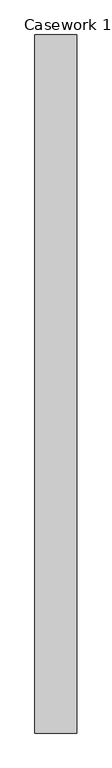
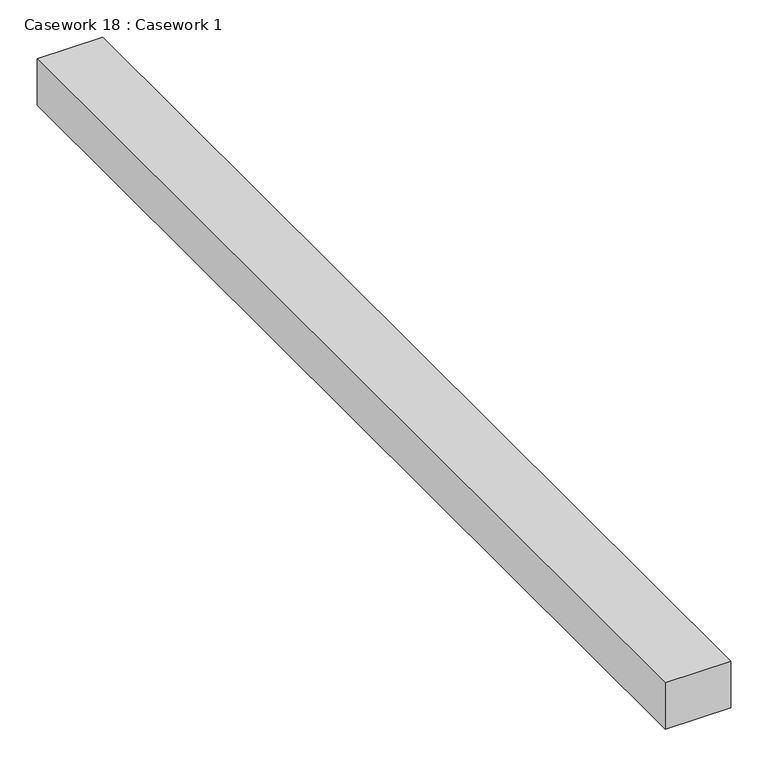
"""IFC4 building model written with IfcOpenShell, lengths in millimetres: furniture geometry, Casework 18 : Casework 1."""

from ifc_helpers import new_model, si_unit, frame, origin, place, context, project, spatial, polyline, outline, extrude, source, transform, mapped, element, save


def casework_18_casework_1_4256c183(model_context):
    return source(origin(), model_context, "Body", "SweptSolid", [
        extrude(outline(polyline([(5395.3559589, 14787.9496924), (5395.3559589, 13098.8496924), (5293.7559589, 13098.8496924), (5293.7559589, 14787.9496924), (5395.3559589, 14787.9496924)])), frame((0.0, 0.0, 3581.4), z_axis=(0.0, 0.0, 1.0), x_axis=(1.0, 0.0, 0.0)), (0.0, 0.0, 1.0), 76.2),
    ])


if __name__ == "__main__":
    model = new_model("IFC4")
    model_context = context("Model", 3, world=origin())
    ifc_project = project(units=[si_unit("LENGTHUNIT", "METRE", prefix="MILLI")], contexts=[model_context])
    site = spatial("IfcSite", under=ifc_project)
    building = spatial("IfcBuilding", under=site)
    placement = place(None, origin())
    casework_18_casework_1_shape = casework_18_casework_1_4256c183(model_context)
    element("IfcFurniture", 1, ObjectType="Casework 18 : Casework 1", at=placement, inside=building, context=model_context, shape_type="MappedRepresentation", body=[
        mapped(casework_18_casework_1_shape, transform((0.0, 0.0, 0.0), x_axis=(1.0, 0.0, 0.0), y_axis=(0.0, 1.0, 0.0), z_axis=(0.0, 0.0, 1.0))),
    ])
    save(model, "model.ifc")

# Revit data of these elements
# Element 1 (IfcFurniture, "Casework 18 : Casework 1")
#   Materials on its faces: "Clad - White"
# Materials
#   "Clad - White": class "Wood", colour RGB 242 242 238, transparency 0, Cost = 0
